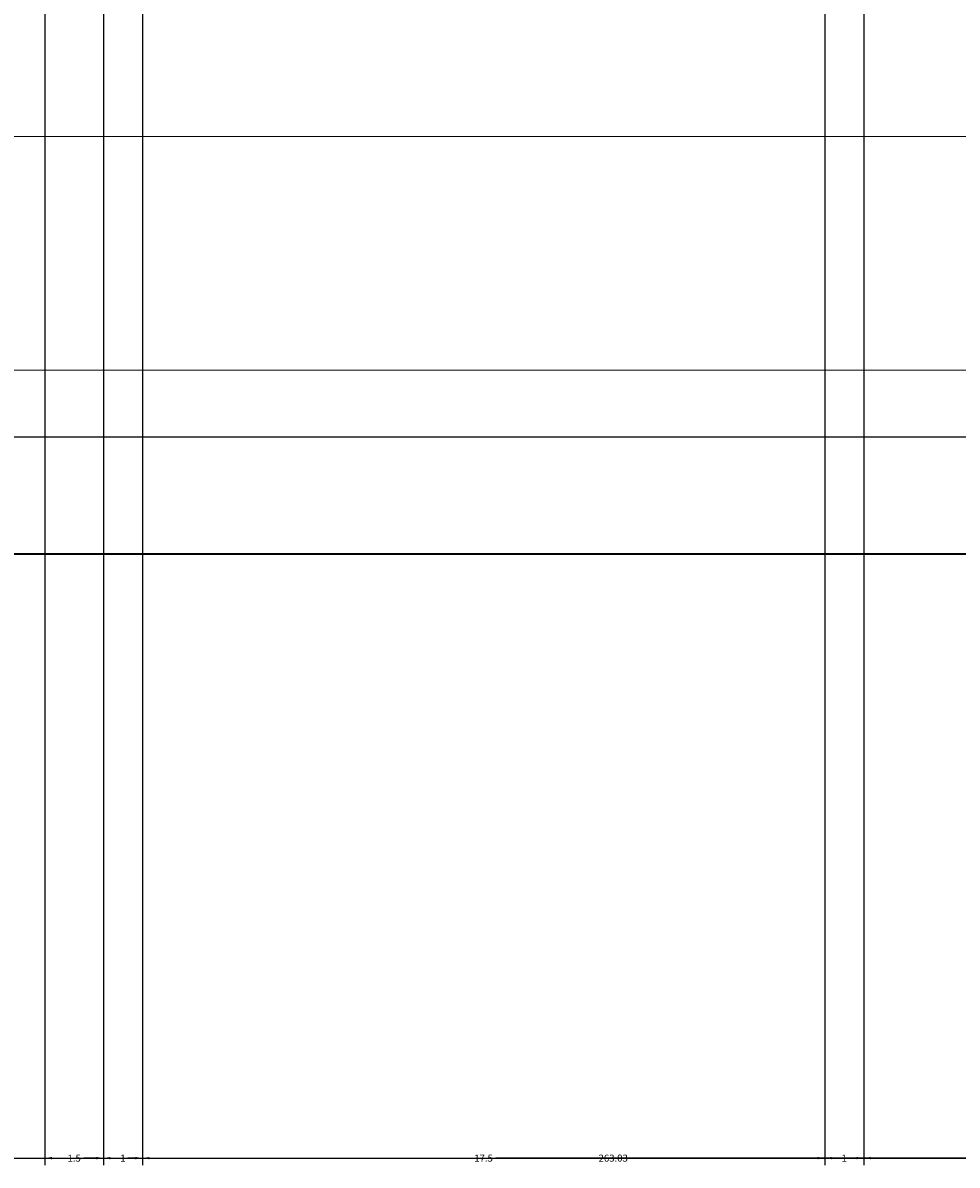
# Model space of a CAD drawing. Units: inches. Extents: x -6 to 289, y -8 to 323.
# Tile 16 of 107: x 126 to 150, y -8 to 21. Entities that reach past the tile are written whole.
import ezdxf

# ---------------------------------------------------------------- set-up
doc = ezdxf.new("R2010")
doc.units = ezdxf.units.IN
doc.header["$MEASUREMENT"] = 0
for name, color, linetype, lineweight in [('A-ANNO-DIMS', 2, 'Continuous', 18), ('A-DOOR', 3, 'Continuous', 25), ('A-ELEV', 7, 'Continuous', 35), ('A-ELEV-PATT', 8, 'Continuous', 13)]:
    doc.layers.add(name, color=color, linetype=linetype, lineweight=lineweight)
doc.styles.get("Standard").update_dxf_attribs({"font": 'arial.ttf'})
doc.dimstyles.get("Standard").update_dxf_attribs({"dimtxt": 0.18, "dimasz": 0.18, "dimexe": 0.18, "dimexo": 0.0625, "dimgap": 0.09, "dimtad": 0, "dimtih": 1, "dimtoh": 1, "dimdec": 4, "dimzin": 0, "dimdsep": 46, "dimtxsty": 'Standard', "dimcen": 0.09, "dimadec": 0, "dimazin": 0, "dimtfac": 1, "dimtdec": 4, "dimtofl": 0, "dimtmove": 0, "dimatfit": 3, "dimfxl": 1, "dimtolj": 1, "dimtzin": 0, "dimarcsym": 0})

# ---------------------------------------------------------------- blocks, each defined once
blk = doc.blocks.new('*D16')
at = {"layer": 'A-ANNO-DIMS', "color": 0, "lineweight": -2, "transparency": 16777216}
for p, q in [((9.943, 68.37), (9.943, -8.391)), ((272.973, 68.37), (272.973, -8.391)), ((10.123, -8.211), (140.993, -8.211)), ((272.793, -8.211), (141.923, -8.211))]:
    blk.add_line(p, q, dxfattribs=at)
at = {"layer": 'A-ANNO-DIMS', "color": 0, "transparency": 16777216}
for points in [[(10.123, -8.181), (10.123, -8.241), (9.943, -8.211)], [(272.793, -8.181), (272.793, -8.241), (272.973, -8.211)]]:
    blk.add_solid(points, dxfattribs=at)
at = {"layer": 'Defpoints', "color": 0, "transparency": 16777216}
for p in [(9.943, 68.432), (272.973, 68.432), (272.973, -8.211)]:
    blk.add_point(p, dxfattribs=at)
at = {"layer": 'A-ANNO-DIMS', "color": 0, "transparency": 16777216, "insert": (141.458, -8.211), "char_height": 0.18, "attachment_point": 5}
blk.add_mtext('\\A1;263.03', dxfattribs=at)
blk = doc.blocks.new('*D28')
at = {"layer": 'A-ANNO-DIMS', "color": 0, "lineweight": -2, "transparency": 16777216}
for p, q in [((128.383, 180.092), (128.383, -8.391)), ((126.883, 178.592), (126.883, -8.391)), ((127.063, -8.211), (127.387, -8.211)), ((128.203, -8.211), (127.88, -8.211))]:
    blk.add_line(p, q, dxfattribs=at)
at = {"layer": 'A-ANNO-DIMS', "color": 0, "transparency": 16777216}
for points in [[(127.063, -8.181), (127.063, -8.241), (126.883, -8.211)], [(128.203, -8.181), (128.203, -8.241), (128.383, -8.211)]]:
    blk.add_solid(points, dxfattribs=at)
at = {"layer": 'Defpoints', "color": 0, "transparency": 16777216}
for p in [(128.383, 180.154), (126.883, 178.654), (128.383, -8.211)]:
    blk.add_point(p, dxfattribs=at)
at = {"layer": 'A-ANNO-DIMS', "color": 0, "transparency": 16777216, "insert": (127.633, -8.211), "char_height": 0.18, "attachment_point": 5}
blk.add_mtext('\\A1;1.5', dxfattribs=at)
blk = doc.blocks.new('*D29')
at = {"layer": 'A-ANNO-DIMS', "color": 0, "lineweight": -2, "transparency": 16777216}
for p, q in [((129.383, 181.092), (129.383, -8.391)), ((128.383, 180.092), (128.383, -8.391)), ((128.563, -8.211), (128.76, -8.211)), ((129.203, -8.211), (129.007, -8.211))]:
    blk.add_line(p, q, dxfattribs=at)
at = {"layer": 'A-ANNO-DIMS', "color": 0, "transparency": 16777216}
for points in [[(128.563, -8.181), (128.563, -8.241), (128.383, -8.211)], [(129.203, -8.181), (129.203, -8.241), (129.383, -8.211)]]:
    blk.add_solid(points, dxfattribs=at)
at = {"layer": 'Defpoints', "color": 0, "transparency": 16777216}
for p in [(129.383, 181.154), (128.383, 180.154), (129.383, -8.211)]:
    blk.add_point(p, dxfattribs=at)
at = {"layer": 'A-ANNO-DIMS', "color": 0, "transparency": 16777216, "insert": (128.883, -8.211), "char_height": 0.18, "attachment_point": 5}
blk.add_mtext('\\A1;1', dxfattribs=at)
blk = doc.blocks.new('*D30')
at = {"layer": 'A-ANNO-DIMS', "color": 0, "lineweight": -2, "transparency": 16777216}
for p, q in [((129.383, 181.092), (129.383, -8.391)), ((146.883, 181.092), (146.883, -8.391)), ((129.563, -8.211), (137.817, -8.211)), ((146.703, -8.211), (138.449, -8.211))]:
    blk.add_line(p, q, dxfattribs=at)
at = {"layer": 'A-ANNO-DIMS', "color": 0, "transparency": 16777216}
for points in [[(129.563, -8.181), (129.563, -8.241), (129.383, -8.211)], [(146.703, -8.181), (146.703, -8.241), (146.883, -8.211)]]:
    blk.add_solid(points, dxfattribs=at)
at = {"layer": 'Defpoints', "color": 0, "transparency": 16777216}
for p in [(129.383, 181.154), (146.883, 181.154), (146.883, -8.211)]:
    blk.add_point(p, dxfattribs=at)
at = {"layer": 'A-ANNO-DIMS', "color": 0, "transparency": 16777216, "insert": (138.133, -8.211), "char_height": 0.18, "attachment_point": 5}
blk.add_mtext('\\A1;17.5', dxfattribs=at)
blk = doc.blocks.new('*D31')
at = {"layer": 'A-ANNO-DIMS', "color": 0, "lineweight": -2, "transparency": 16777216}
for p, q in [((146.883, 181.092), (146.883, -8.391)), ((147.883, 181.092), (147.883, -8.391)), ((147.063, -8.211), (147.26, -8.211)), ((147.703, -8.211), (147.507, -8.211))]:
    blk.add_line(p, q, dxfattribs=at)
at = {"layer": 'A-ANNO-DIMS', "color": 0, "transparency": 16777216}
for points in [[(147.063, -8.181), (147.063, -8.241), (146.883, -8.211)], [(147.703, -8.181), (147.703, -8.241), (147.883, -8.211)]]:
    blk.add_solid(points, dxfattribs=at)
at = {"layer": 'Defpoints', "color": 0, "transparency": 16777216}
for p in [(146.883, 181.154), (147.883, 181.154), (147.883, -8.211)]:
    blk.add_point(p, dxfattribs=at)
at = {"layer": 'A-ANNO-DIMS', "color": 0, "transparency": 16777216, "insert": (147.383, -8.211), "char_height": 0.18, "attachment_point": 5}
blk.add_mtext('\\A1;1', dxfattribs=at)
blk = doc.blocks.new('*D32')
at = {"layer": 'A-ANNO-DIMS', "color": 0, "lineweight": -2, "transparency": 16777216}
for p, q in [((147.883, 181.092), (147.883, -8.391)), ((166.383, 181.092), (166.383, -8.391)), ((148.063, -8.211), (156.817, -8.211)), ((166.203, -8.211), (157.449, -8.211))]:
    blk.add_line(p, q, dxfattribs=at)
at = {"layer": 'A-ANNO-DIMS', "color": 0, "transparency": 16777216}
for points in [[(148.063, -8.181), (148.063, -8.241), (147.883, -8.211)], [(166.203, -8.181), (166.203, -8.241), (166.383, -8.211)]]:
    blk.add_solid(points, dxfattribs=at)
at = {"layer": 'Defpoints', "color": 0, "transparency": 16777216}
for p in [(147.883, 181.154), (166.383, 181.154), (166.383, -8.211)]:
    blk.add_point(p, dxfattribs=at)
at = {"layer": 'A-ANNO-DIMS', "color": 0, "transparency": 16777216, "insert": (157.133, -8.211), "char_height": 0.18, "attachment_point": 5}
blk.add_mtext('\\A1;18.5', dxfattribs=at)
blk = doc.blocks.new('*D68')
at = {"layer": 'A-ANNO-DIMS', "color": 0, "lineweight": -2, "transparency": 16777216}
for p, q in [((124.008, 10.226), (124.008, -8.391)), ((184.124, 10.226), (184.124, -8.391)), ((124.188, -8.211), (153.673, -8.211)), ((183.944, -8.211), (154.459, -8.211))]:
    blk.add_line(p, q, dxfattribs=at)
at = {"layer": 'A-ANNO-DIMS', "color": 0, "transparency": 16777216}
for points in [[(124.188, -8.181), (124.188, -8.241), (124.008, -8.211)], [(183.944, -8.181), (183.944, -8.241), (184.124, -8.211)]]:
    blk.add_solid(points, dxfattribs=at)
at = {"layer": 'Defpoints', "color": 0, "transparency": 16777216}
for p in [(124.008, 10.289), (184.124, 10.289), (184.124, -8.211)]:
    blk.add_point(p, dxfattribs=at)
at = {"layer": 'A-ANNO-DIMS', "color": 0, "transparency": 16777216, "insert": (154.066, -8.211), "char_height": 0.18, "attachment_point": 5}
blk.add_mtext('\\A1;60.12', dxfattribs=at)

msp = doc.modelspace()

# ---------------------------------------------------------------- hatches: boundary and pattern name
at = {"layer": 'A-ELEV-PATT'}
h = msp.add_hatch(dxfattribs=at)
h.set_pattern_fill('_USER', color=256, scale=6, pattern_type=0)
h.set_pattern_definition([(0, (0, 0), (0, 6), [])])
h.paths.add_polyline_path([(184.1244, 48.0851), (124.008, 48.0851), (124.008, 10.2888), (184.1244, 10.2888)])
h.paths.add_polyline_path([(244.2408, 48.0851), (186.3604, 48.0851), (186.3604, 10.2888), (244.2408, 10.2888)])
h.paths.add_polyline_path([(208.2918, 114.2795), (190.7918, 114.2795), (190.7918, 71.2795), (208.2918, 71.2795)])
h.paths.add_polyline_path([(227.7918, 114.2795), (209.2918, 114.2795), (209.2918, 71.2795), (227.7918, 71.2795)])
h.paths.add_polyline_path([(211.2918, 224.3887), (190.7918, 224.3887), (190.7918, 162.3484), (211.2918, 162.3484)])
h.paths.add_polyline_path([(233.7918, 224.3887), (212.2918, 224.3887), (212.2918, 162.3484), (233.7918, 162.3484)])
h.paths.add_polyline_path([(166.3835, 224.154), (147.8835, 224.154), (147.8835, 181.154), (166.3835, 181.154)])
h.paths.add_polyline_path([(146.8835, 224.154), (129.3835, 224.154), (129.3835, 181.154), (146.8835, 181.154)])

# ---------------------------------------------------------------- linework, layer by layer
at = {"layer": 'A-DOOR'}
for points in [[(121.008, 51.0851), (247.2408, 51.0851), (247.2408, 7.2888), (121.008, 7.2888)], [(124.008, 48.0851), (244.2408, 48.0851), (244.2408, 10.2888), (124.008, 10.2888)]]:
    msp.add_lwpolyline(points, close=True, dxfattribs=at)
at = {"layer": 'A-ELEV'}
msp.add_line((19.1638, 7.2888), (271.1638, 7.2888), dxfattribs=at)

# ---------------------------------------------------------------- dimensions: what is measured, and where the dimension line sits
at = {"layer": 'A-ANNO-DIMS'}
for base, p1, p2, override, picture, middle in [((129.3835, -8.2112), (128.3835, 180.154), (129.3835, 181.154), {"dimdec": 0, "dimlfac": 1, "dimrnd": 0, "dimzin": 0, "dimdsep": 46, "dimlunit": 2}, '*D29', (128.8835, -8.2112)), ((146.8835, -8.2112), (129.3835, 181.154), (146.8835, 181.154), {"dimdec": 1, "dimlfac": 1, "dimrnd": 0, "dimzin": 0, "dimdsep": 46, "dimlunit": 2}, '*D30', (138.1335, -8.2112)), ((147.8835, -8.2112), (146.8835, 181.154), (147.8835, 181.154), {"dimdec": 0, "dimlfac": 1, "dimrnd": 0, "dimzin": 0, "dimdsep": 46, "dimlunit": 2}, '*D31', (147.3835, -8.2112)), ((166.3835, -8.2112), (147.8835, 181.154), (166.3835, 181.154), {"dimdec": 1, "dimlfac": 1, "dimrnd": 0, "dimzin": 0, "dimdsep": 46, "dimlunit": 2}, '*D32', (157.1335, -8.2112)), ((128.3835, -8.2112), (126.8835, 178.654), (128.3835, 180.154), {"dimdec": 1, "dimlfac": 1, "dimrnd": 0, "dimzin": 0, "dimdsep": 46, "dimlunit": 2}, '*D28', (127.6335, -8.2112)), ((272.9733, -8.2112), (9.943, 68.4322), (272.9733, 68.4322), {"dimdec": 2, "dimlfac": 1, "dimrnd": 0, "dimzin": 0, "dimdsep": 46, "dimlunit": 2}, '*D16', (141.4581, -8.2112)), ((184.1244, -8.2112), (124.008, 10.2888), (184.1244, 10.2888), {"dimdec": 2, "dimlfac": 1, "dimrnd": 0, "dimzin": 0, "dimdsep": 46, "dimlunit": 2}, '*D68', (154.0662, -8.2112))]:
    dim = msp.add_linear_dim(base=base, p1=p1, p2=p2, dimstyle='Standard', override=override, dxfattribs=at)
    dim.commit()
    dim.dimension.update_dxf_attribs({"geometry": picture, "text_midpoint": middle})

doc.saveas('drawing.dxf')
